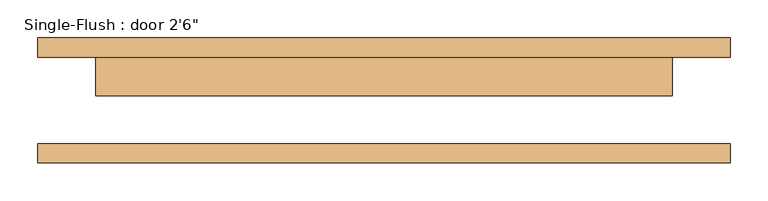
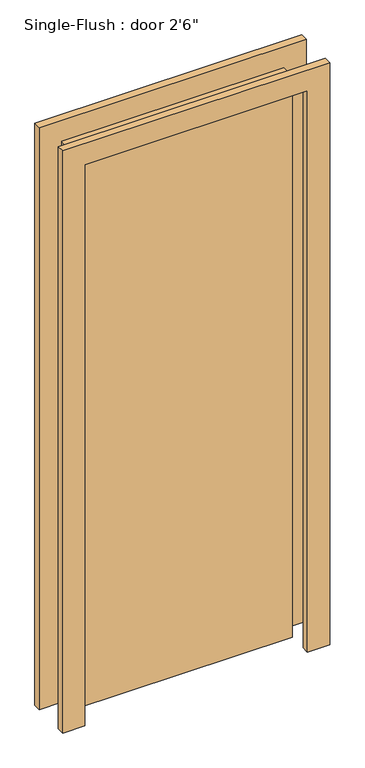
"""IFC4 building model written with IfcOpenShell, lengths in millimetres: door geometry."""

from ifc_helpers import new_model, si_unit, frame, origin, origin_with_axes, place, context, project, spatial, polyline, outline, extrude, source, transform, mapped, element, save


def door_d8f5dbb5(model_context):
    return source(origin(), model_context, "Body", "SweptSolid", [
        extrude(outline(polyline([(2108.2, -457.2), (0.0, -457.2), (0.0, -381.0), (2032.0, -381.0), (2032.0, 381.0), (0.0, 381.0), (0.0, 457.2), (2108.2, 457.2), (2108.2, -457.2)])), frame((0.0, 57.15, 0.0), z_axis=(0.0, 1.0, 0.0), x_axis=(0.0, 0.0, 1.0)), (0.0, 0.0, 1.0), 25.4),
        extrude(outline(polyline([(2108.2, 457.2), (2108.2, -457.2), (0.0, -457.2), (0.0, -381.0), (2032.0, -381.0), (2032.0, 381.0), (0.0, 381.0), (0.0, 457.2), (2108.2, 457.2)])), frame((0.0, -82.55, 0.0), z_axis=(0.0, 1.0, 0.0), x_axis=(0.0, 0.0, 1.0)), (0.0, 0.0, 1.0), 25.4),
        extrude(outline(polyline([(381.0, 6.35), (-381.0, 6.35), (-381.0, 57.15), (381.0, 57.15), (381.0, 6.35)])), origin_with_axes(), (0.0, 0.0, 1.0), 2032.0),
    ])


if __name__ == "__main__":
    model = new_model("IFC4")
    model_context = context("Model", 3, world=origin())
    ifc_project = project(units=[si_unit("LENGTHUNIT", "METRE", prefix="MILLI")], contexts=[model_context])
    site = spatial("IfcSite", under=ifc_project)
    building = spatial("IfcBuilding", under=site)
    placement = place(None, origin())
    door_shape = door_d8f5dbb5(model_context)
    element("IfcDoor", 1, ObjectType="Single-Flush : door 2'6\"", at=placement, inside=building, context=model_context, shape_type="MappedRepresentation", body=[
        mapped(door_shape, transform((0.0, 0.0, 0.0), x_axis=(1.0, 0.0, 0.0), y_axis=(0.0, 1.0, 0.0), z_axis=(0.0, 0.0, 1.0))),
    ])
    save(model, "model.ifc")

# Revit data of these elements
# Type "Single-Flush : door 2'6\""
#   Type Mark = "10"
#   Construction Type Id = "MDOOR"
#   Assembly Code = "C1020"
#   Analytic Construction = "Metal"
#   Thickness = 0' - 2"
#   Heat Transfer Coefficient (U) = 0.651978 BTU/(h·ft²·°F)
#   Height = 6' - 8"
#   Trim Projection Ext = 0' - 1"
#   Trim Projection Int = 0' - 1"
#   Trim Width = 0' - 3"
#   Width = 2' - 6"
#   Define Thermal Properties by = 1
#   Door Material = Door - Panel
#   Frame Material = Door - Frame
#   Visual Light Transmittance = 0
#   Solar Heat Gain Coefficient = 0
#   Function = (empty or 0)
#   Wall Closure = (empty or 0)
# Element 1 (IfcDoor, "Single-Flush : door 2'6\"")
#   Materials on its faces: "Door - Frame", "Door - Panel"
# Materials
#   "Door - Panel": class "Wood", colour RGB 210 159 95, transparency 0, Cost = 0
#   "Door - Frame": colour RGB 118 70 51, transparency 0, Cost = 0
